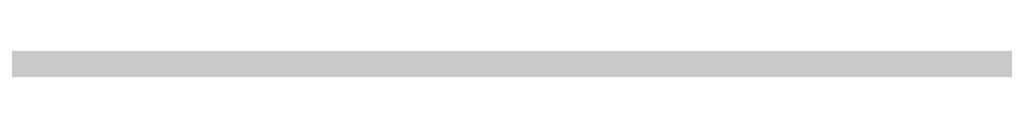
# Model space of a CAD drawing. Units: inches. Extents: x 2091 to 2899, y 967 to 2217.
# Tile 198 of 256: x 2203.18039 to 2203.25707, y 1152.2479 to 1152.24874. Entities that reach past the tile are written whole.
import ezdxf

# ---------------------------------------------------------------- set-up
doc = ezdxf.new("R2010")
doc.units = ezdxf.units.IN
doc.layers.add('A-WALL-PATT', color=141, linetype='Continuous', lineweight=13, true_color=0xadddf7)

msp = doc.modelspace()

# ---------------------------------------------------------------- hatches: boundary and pattern name
at = {"layer": 'A-WALL-PATT'}
h = msp.add_hatch(color=256, dxfattribs=at)
h.dxf.hatch_style = 1
h.paths.add_polyline_path([(2803.143603, 2050.919059), (2203.143603, 2050.919059), (2203.143603, 1090.919059), (2803.143603, 1090.919059)])
h.paths.add_polyline_path([(2635.79885, 1147.540465), (2674.524052, 1147.540465, 0.376086), (2678.529665, 1152.880202), (2678.529665, 1159.556473, 0.333335), (2674.524319, 1163.561846), (2674.524319, 1163.56185), (2674.524319, 1192.93439), (2635.805971, 1192.93439), (2597.087622, 1192.93439), (2597.087622, 1163.561846, 0.333335), (2593.082276, 1159.556473), (2593.082276, 1152.880202, 0.376086), (2597.087889, 1147.540465)], flags=0)
h.paths.add_polyline_path([(2436.010433, 1278.240778, 0.000483), (2435.952643, 1278.215027, -0.001328), (2435.935625, 1278.111693, -0.001711), (2436.11644, 1278.040758, 0.002185)], flags=0)
h.paths.add_polyline_path([(2794.143603, 1143.419059), (2794.143603, 1347.419059), (2543.370171, 1347.419059), (2543.370171, 1351.919059), (2794.143603, 1351.919059), (2794.143603, 1392.713555), (2793.947398, 1392.713555), (2793.947398, 1473.5369), (2794.143603, 1473.5369), (2794.143603, 1531.919059), (2650.143603, 1531.919059), (2650.143603, 1536.419059), (2794.143603, 1536.419059), (2794.143603, 1692.419059), (2609.375609, 1692.419059), (2609.375609, 1644.419059), (2604.875609, 1644.419059), (2604.875609, 1744.919059), (2609.375609, 1744.919059), (2609.375609, 1696.919059), (2794.143603, 1696.919059), (2794.143603, 1780.919059), (2609.643603, 1780.919059), (2493.875609, 1780.919059), (2493.875609, 1785.419059), (2609.643603, 1785.419059), (2794.143603, 1785.419059), (2794.143603, 1847.938821), (2793.951222, 1847.938821), (2793.951222, 1928.762166), (2794.143603, 1928.762166), (2794.143603, 1941.419059), (2614.143603, 1941.419059), (2614.143603, 1821.419059), (2609.643603, 1821.419059), (2609.643603, 1941.419059), (2392.143603, 1941.419059), (2392.143603, 1819.919059), (2387.643603, 1819.919059), (2387.643603, 1941.419059), (2212.143603, 1941.419059), (2212.143603, 1783.919059), (2392.143603, 1783.919059), (2392.143603, 1780.919059), (2212.143603, 1780.919059), (2212.143603, 1629.419059), (2387.643603, 1629.419059), (2387.643603, 1744.919059), (2392.143603, 1744.919059), (2392.143603, 1627.919059), (2317.143603, 1627.919059), (2317.143603, 1551.419059), (2317.143603, 1536.419059), (2459.383591, 1536.419059), (2459.383591, 1602.39648), (2463.883591, 1602.39648), (2463.883591, 1531.919059), (2456.643603, 1531.919059), (2456.643603, 1529.919059), (2452.143603, 1529.919059), (2452.143603, 1531.919059), (2312.643603, 1531.919059), (2312.643603, 1551.419059), (2306.143603, 1551.419059), (2306.143603, 1555.919059), (2308.143603, 1555.919059), (2308.143603, 1551.419059), (2312.643603, 1551.419059), (2312.643603, 1627.919059), (2212.143603, 1627.919059), (2212.143603, 1555.919059), (2270.143603, 1555.919059), (2270.143603, 1551.419059), (2212.143603, 1551.419059), (2212.143603, 1351.919059), (2272.143603, 1351.919059), (2272.143603, 1347.419059), (2212.143603, 1347.419059), (2212.143603, 1275.419059), (2308.143603, 1275.419059), (2308.143603, 1351.919059), (2452.143603, 1351.919059), (2452.143603, 1493.919059), (2456.643603, 1493.919059), (2456.643603, 1347.419059), (2312.643603, 1347.419059), (2312.643603, 1270.919059), (2212.143603, 1270.919059), (2212.143603, 1099.919059), (2281.237523, 1099.919059), (2282.871041, 1110.913803), (2282.008341, 1116.996603), (2278.557741, 1121.420403), (2268.205641, 1128.056203), (2272.087641, 1128.056203), (2273.812941, 1131.927003), (2279.420341, 1134.691903), (2285.027841, 1135.244903), (2287.615841, 1137.456803), (2288.047141, 1138.009803), (2289.341141, 1140.774703), (2291.066541, 1139.668703), (2292.360541, 1135.244903), (2295.379841, 1136.903803), (2296.242541, 1135.797903), (2297.105241, 1133.033003), (2300.124641, 1138.009803), (2303.143941, 1138.009803), (2304.437941, 1135.797903), (2303.143941, 1133.586003), (2306.594641, 1134.691903), (2307.888741, 1133.033003), (2310.908041, 1135.244903), (2313.927441, 1134.138903), (2315.62686, 1132.427102), (2308.320041, 1117.549603), (2290.203841, 1109.807903), (2288.909841, 1103.172103), (2289.272309, 1099.919059), (2434.918227, 1099.919059), (2431.593227, 1124.788059), (2429.930227, 1169.553059), (2430.927185, 1240.519694), (2435.658926, 1238.186126), (2437.135227, 1196.554059), (2438.798227, 1143.973059), (2442.678227, 1111.998059), (2446.558227, 1099.919059), (2794.143603, 1099.919059), (2794.143603, 1138.919059), (2548.032447, 1138.919059), (2548.032447, 1143.419059), (2548.032447, 1148.819059), (2546.668457, 1148.031559), (2528.685692, 1179.178622, 0.256256), (2512.032447, 1148.819059), (2512.032447, 1143.419059), (2512.032447, 1138.919059), (2507.532447, 1138.919059), (2507.532447, 1143.419059), (2507.532447, 1148.819059, 0.256256), (2490.879202, 1179.178622), (2472.896437, 1148.031559), (2471.532447, 1148.819059), (2471.532447, 1143.419059), (2467.032447, 1143.419059), (2467.032447, 1269.945786, 0.039061), (2460.909987, 1273.580059), (2467.032447, 1273.580059), (2467.032447, 1286.325364, 0.014511), (2465.216194, 1286.761905), (2467.032447, 1287.052576), (2467.032447, 1323.419059), (2471.532447, 1323.419059), (2471.532447, 1148.819059), (2489.532447, 1179.995973), (2490.896437, 1179.208473), (2490.879202, 1179.178622, -0.256256), (2507.532447, 1148.819059), (2507.532447, 1143.419059), (2512.032447, 1143.419059), (2512.032447, 1148.819059, -0.256256), (2528.685692, 1179.178622), (2528.668457, 1179.208473), (2530.032447, 1179.995973), (2548.032447, 1148.819059), (2548.032447, 1143.419059)], flags=16)
h.paths.add_polyline_path([(2607.768546, 1200.945083), (2607.768546, 1265.030625), (2597.087622, 1281.052011), (2619.784585, 1281.052011), (2627.795278, 1337.12686), (2635.79885, 1337.12686), (2643.816663, 1337.12686), (2651.827356, 1281.052011), (2674.524319, 1281.052011), (2663.843395, 1265.030625), (2663.843395, 1200.945083), (2635.805971, 1200.945083)], flags=0)
edge = h.paths.add_edge_path(flags=0)
edge.add_ellipse((13303.896215, 1272.998725), major_axis=(-10595.31304, 0.000001), ratio=0.842303870086, start_angle=0.6282372191, end_angle=0.6465540999, ccw=False)
edge.add_ellipse((2711.70045, 1156.852678), major_axis=(2.219769, 0), ratio=0.84230387, start_angle=111.535244, end_angle=180.628237, ccw=False)
edge.add_ellipse((13303.156292, 1272.998725), major_axis=(-10593.026306, 0), ratio=0.842303869544, start_angle=0.5282714718, end_angle=0.6465540971, ccw=False)
edge.add_line((2710.764596, 1175.333295), (2710.129986, 1175.333295))
edge.add_ellipse((2710.129986, 1176.579775), major_axis=(1.479846, 0), ratio=0.84230387, start_angle=180, end_angle=270, ccw=False)
edge.add_line((2708.65014, 1176.579775), (2708.65014, 1200.782914))
edge.add_ellipse((2710.129986, 1200.782914), major_axis=(1.479846, 0), ratio=0.84230387, start_angle=90, end_angle=180, ccw=False)
edge.add_line((2710.129986, 1202.029394), (2710.465075, 1202.029394))
edge.add_ellipse((13303.156292, 1272.998725), major_axis=(-10593.026306, 0), ratio=0.842303869544, start_angle=-0.0902290886, end_angle=0.3838667788, ccw=False)
edge.add_ellipse((2710.129986, 1290.927031), major_axis=(-1.479846, 0), ratio=0.84230387, start_angle=0, end_angle=90, ccw=False)
edge.add_line((2708.65014, 1290.927031), (2708.65014, 1315.13017))
edge.add_ellipse((2710.129986, 1315.13017), major_axis=(-1.479846, 0), ratio=0.84230387, start_angle=-90, end_angle=0, ccw=False)
edge.add_line((2710.129986, 1316.37665), (2710.706314, 1316.37665))
edge.add_ellipse((3238.40172, 1296.289566), major_axis=(528.234, 0), ratio=0.8423038695, start_angle=176.34957241, end_angle=177.82004969, ccw=False)
edge.add_ellipse((2775.063043, 1071.450696), major_axis=(313.307761, 0), ratio=0.8423038695, start_angle=102.12596555, end_angle=103.78052899, ccw=False)
edge.add_ellipse((2775.063043, 1078.305698), major_axis=(-305.302891, 0), ratio=0.8423038695, start_angle=-79.790461, end_angle=-77.55537271, ccw=False)
edge.add_ellipse((2695.141767, 1541.975383), major_axis=(-250.960216, 0), ratio=0.8423038695, start_angle=99.25656601, end_angle=102.55493264)
edge.add_line((2741.410326, 1334.214255), (2747.132545, 1337.378477))
edge.add_ellipse((2747.538616, 1336.857478), major_axis=(-0.739923, 0), ratio=0.8423039, start_angle=270, end_angle=307.93313, ccw=False)
edge.add_ellipse((2747.538616, 1336.857478), major_axis=(-0.739923, 0), ratio=0.8423039, start_angle=232.06687, end_angle=270, ccw=False)
edge.add_line((2747.944687, 1337.378477), (2753.666906, 1334.214255))
edge.add_ellipse((2799.935466, 1541.975383), major_axis=(250.960216, 0), ratio=0.8423038695, start_angle=257.44506736, end_angle=260.74343399)
edge.add_ellipse((2720.014189, 1078.305698), major_axis=(305.302891, 0), ratio=0.8423038695, start_angle=77.55537271, end_angle=79.790461, ccw=False)
edge.add_ellipse((2720.014189, 1071.450696), major_axis=(-313.307761, 0), ratio=0.8423038695, start_angle=256.21947101, end_angle=257.87403445, ccw=False)
edge.add_ellipse((2256.675512, 1296.289566), major_axis=(-528.234, 0), ratio=0.8423038695, start_angle=182.17995031, end_angle=183.65042759, ccw=False)
edge.add_line((2784.370918, 1316.37665), (2784.947247, 1316.37665))
edge.add_ellipse((2784.947247, 1315.13017), major_axis=(1.479846, 0), ratio=0.84230387, start_angle=0, end_angle=90, ccw=False)
edge.add_line((2786.427093, 1315.13017), (2786.427093, 1290.927031))
edge.add_ellipse((2784.947247, 1290.927031), major_axis=(1.479846, 0), ratio=0.84230387, start_angle=270, end_angle=360, ccw=False)
edge.add_ellipse((-7808.07906, 1272.998725), major_axis=(10593.026306, 0), ratio=0.842303869544, start_angle=-0.3838667788, end_angle=0.0902290886, ccw=False)
edge.add_line((2784.612157, 1202.029394), (2784.947247, 1202.029394))
edge.add_ellipse((2784.947247, 1200.782914), major_axis=(1.479846, 0), ratio=0.84230387, start_angle=0, end_angle=90, ccw=False)
edge.add_line((2786.427093, 1200.782914), (2786.427093, 1176.579775))
edge.add_ellipse((2784.947247, 1176.579775), major_axis=(-1.479846, 0), ratio=0.84230387, start_angle=90, end_angle=180, ccw=False)
edge.add_line((2784.947247, 1175.333295), (2784.312636, 1175.333295))
edge.add_ellipse((-7808.07906, 1272.998725), major_axis=(10593.026306, 0), ratio=0.842303869544, start_angle=-0.6186431963, end_angle=-0.5282714718, ccw=False)
edge.add_ellipse((2783.376783, 1156.852678), major_axis=(-2.219769, 0), ratio=0.84230387, start_angle=179.371763, end_angle=248.464757, ccw=False)
edge.add_ellipse((-7808.818983, 1272.998725), major_axis=(-10595.31304, 0.000004), ratio=0.842303865762, start_angle=179.3534459226, end_angle=179.3717628034, ccw=False)
edge.add_ellipse((2780.297303, 1153.500793), major_axis=(-5.246426, 0), ratio=0.84230387, start_angle=90, end_angle=179.353446, ccw=False)
edge.add_line((2780.297303, 1149.081708), (2714.77993, 1149.081708))
edge.add_ellipse((2714.77993, 1153.500793), major_axis=(5.246426, 0), ratio=0.84230387, start_angle=180.646554, end_angle=270, ccw=False)
edge = h.paths.add_edge_path(flags=0)
edge.add_line((2718.187367, 1151.007833), (2718.187367, 1170.472364))
edge.add_ellipse((2721.14706, 1170.472364), major_axis=(-2.959692, 0), ratio=0.84230387, start_angle=-90, end_angle=0, ccw=False)
edge.add_line((2721.14706, 1172.965324), (2773.930173, 1172.965324))
edge.add_ellipse((2773.930173, 1170.472364), major_axis=(-2.959692, 0), ratio=0.84230387, start_angle=180, end_angle=270, ccw=False)
edge.add_line((2776.889865, 1170.472364), (2776.889865, 1151.007833))
edge.add_line((2776.889865, 1151.007833), (2718.187367, 1151.007833))
edge = h.paths.add_edge_path(flags=0)
edge.add_line((2718.187367, 1180.23415), (2718.187367, 1199.057834))
edge.add_ellipse((2747.538616, 1320.39864), major_axis=(147.017924, 0), ratio=0.8423038695, start_angle=256.40186531, end_angle=283.59813469)
edge.add_line((2776.889865, 1199.057834), (2776.889865, 1180.23415))
edge.add_ellipse((2747.538616, 1301.574956), major_axis=(147.017924, 0), ratio=0.8423038695, start_angle=256.40186531, end_angle=283.59813469, ccw=False)
edge = h.paths.add_edge_path(flags=0)
edge.add_ellipse((13303.156292, 1272.998725), major_axis=(-10591.54646, 0), ratio=0.842303869555, start_angle=0.0555943135, end_angle=0.3777641939, ccw=False)
edge.add_line((2711.616859, 1262.72171), (2715.667408, 1249.495396))
edge.add_ellipse((6413.891963, 1241.691919), major_axis=(-3698.236159, 0), ratio=0.84230386955, start_angle=-0.120897369, end_angle=0.364076349)
edge.add_line((2715.761038, 1218.192455), (2711.934307, 1203.167361))
edge = h.paths.add_edge_path(flags=0)
edge.add_line((2718.187367, 1251.074566), (2716.002485, 1267.450435))
edge.add_ellipse((2742.151175, 1202.18954), major_axis=(81.772585, 0), ratio=0.84230387, start_angle=94.27742096, end_angle=111.8349538, ccw=False)
edge.add_line((2737.009748, 1270.930626), (2758.067484, 1270.930626))
edge.add_ellipse((2752.926058, 1202.18954), major_axis=(81.772585, 0), ratio=0.84230387, start_angle=68.1650462, end_angle=85.72257904, ccw=False)
edge.add_line((2779.074747, 1267.450435), (2776.889865, 1251.074566))
edge.add_ellipse((2750.338059, 1187.885356), major_axis=(79.579664, 0), ratio=0.84230387, start_angle=67.20808512, end_angle=85.1299304)
edge.add_line((2756.034656, 1254.743656), (2739.042576, 1254.743656))
edge.add_ellipse((2744.739174, 1187.885356), major_axis=(79.579664, 0), ratio=0.84230387, start_angle=94.8700696, end_angle=112.79191488)
edge = h.paths.add_edge_path(flags=0)
edge.add_line((2783.142926, 1203.167361), (2779.316194, 1218.192455))
edge.add_ellipse((-918.81473, 1241.691919), major_axis=(3698.236159, 0), ratio=0.84230386955, start_angle=-0.364076349, end_angle=0.120897369)
edge.add_line((2779.409825, 1249.495396), (2783.460373, 1262.72171))
edge.add_ellipse((-7808.07906, 1272.998725), major_axis=(-10591.54646, 0), ratio=0.84230386954, start_angle=179.6222358061, end_angle=179.9444056865, ccw=False)
edge = h.paths.add_edge_path(flags=0)
edge.add_ellipse((2734.200892, 1286.69044), major_axis=(-0.356609, 6.340078), ratio=0.60383358, start_angle=89.0020143, end_angle=253.657408, ccw=False)
edge.add_line((2730.369001, 1286.541806), (2730.369001, 1301.35198))
edge.add_line((2730.369001, 1301.35198), (2735.913311, 1305.214803))
edge.add_ellipse((2736.384917, 1304.734561), major_axis=(0.739923, 0), ratio=0.8423039, start_angle=90, end_angle=134.480211, ccw=False)
edge.add_line((2736.384917, 1305.357801), (2738.032783, 1305.357801))
edge.add_line((2738.032783, 1305.357801), (2738.032783, 1307.707927))
edge.add_ellipse((2794.201642, 1307.707927), major_axis=(56.168859, 0), ratio=0.84230387, start_angle=150.5614304, end_angle=180, ccw=False)
edge.add_ellipse((2700.875591, 1307.707927), major_axis=(-56.168859, 0), ratio=0.84230387, start_angle=180, end_angle=209.4385696, ccw=False)
edge.add_line((2757.04445, 1307.707927), (2757.04445, 1305.357801))
edge.add_line((2757.04445, 1305.357801), (2758.692316, 1305.357801))
edge.add_ellipse((2758.692316, 1304.734561), major_axis=(-0.739923, 0), ratio=0.8423039, start_angle=225.519789, end_angle=270, ccw=False)
edge.add_line((2759.163922, 1305.214803), (2764.708231, 1301.35198))
edge.add_line((2764.708231, 1301.35198), (2764.708231, 1286.541806))
edge.add_ellipse((2760.87634, 1286.69044), major_axis=(0.356609, 6.340078), ratio=0.60383358, start_angle=106.342592, end_angle=270.9979857, ccw=False)
edge.add_line((2757.04445, 1285.79709), (2757.04445, 1307.707927))
edge.add_ellipse((2700.875591, 1307.707927), major_axis=(-56.168859, 0), ratio=0.84230387, start_angle=180, end_angle=209.4385696)
edge.add_ellipse((2794.201642, 1307.707927), major_axis=(56.168859, 0), ratio=0.84230387, start_angle=150.5614304, end_angle=180)
edge.add_line((2738.032783, 1307.707927), (2738.032783, 1285.79709))
h.paths.add_polyline_path([(2417.812273, 1104.449704), (2413.492273, 1102.529704), (2410.612273, 1103.969704), (2409.172273, 1106.369704), (2407.252273, 1107.329704), (2406.292273, 1109.729704), (2405.332273, 1114.049704), (2405.332273, 1117.889704), (2406.292273, 1120.129704), (2407.252273, 1119.809704), (2408.848322, 1118.327658), (2410.173945, 1119.42417), (2410.211273, 1120.405704), (2411.040731, 1121.419054), (2410.699273, 1119.858704), (2410.173945, 1119.42417), (2410.088452, 1117.176109), (2411.132836, 1116.206324), (2413.972273, 1119.329704), (2416.852273, 1120.769704), (2416.869721, 1120.798784), (2417.035071, 1119.405116), (2417.896213, 1118.143384), (2418.292273, 1118.369704), (2419.544447, 1120.039269), (2419.360915, 1118.387487), (2419.032108, 1119.356151), (2418.398939, 1118.511926), (2419.252273, 1114.529704), (2418.794091, 1107.198795)], flags=0)
h.paths.add_polyline_path([(2508.870171, 1347.419059), (2508.370171, 1347.419059), (2508.370171, 1351.919059), (2508.870171, 1351.919059)], flags=0)
h.paths.add_polyline_path([(2473.370171, 1347.419059), (2472.370171, 1347.419059), (2467.870171, 1347.419059), (2467.870171, 1455.419059), (2472.370171, 1455.419059), (2472.370171, 1352.419059), (2473.370171, 1352.419059)], flags=0)
h.paths.add_polyline_path([(2352.106244, 1217.446197), (2349.226244, 1218.886197), (2347.786244, 1221.286197), (2345.866244, 1222.246197), (2344.906244, 1224.646197), (2343.946244, 1228.966197), (2343.946244, 1232.806197), (2344.906244, 1235.046197), (2345.866244, 1234.726197), (2347.462293, 1233.244152), (2348.787916, 1234.340663), (2348.825244, 1235.322197), (2349.654702, 1236.335547), (2349.313244, 1234.775197), (2348.787916, 1234.340663), (2348.702423, 1232.092603), (2349.746807, 1231.122817), (2352.586244, 1234.246197), (2355.466244, 1235.686197), (2355.483692, 1235.715277), (2355.649043, 1234.321609), (2356.510185, 1233.059877), (2356.906244, 1233.286197), (2358.158418, 1234.955762), (2357.974887, 1233.30398), (2357.646079, 1234.272644), (2357.012911, 1233.428419), (2357.866244, 1229.446197), (2357.408062, 1222.115288), (2356.426244, 1219.366197)], flags=0)
h.paths.add_polyline_path([(2348.2968, 1112.22442), (2347.0138, 1112.31042), (2345.5298, 1114.12742), (2345.7318, 1115.85842), (2346.8118, 1116.98242), (2346.8118, 1114.64642), (2345.8668, 1114.21442), (2346.8798, 1114.30042)], flags=0)
h.paths.add_polyline_path([(2347.0138, 1110.92642), (2346.2718, 1110.49342), (2346.6098, 1111.18642)], flags=0)
h.paths.add_polyline_path([(2345.8668, 1118.19442), (2345.5298, 1117.32942), (2343.7078, 1118.02142), (2344.3828, 1118.62642)], flags=0)
h.paths.add_polyline_path([(2346.6768, 1109.28242), (2346.0698, 1108.07142), (2345.8668, 1110.06142)], flags=0)
h.paths.add_polyline_path([(2345.0568, 1119.75142), (2343.6398, 1119.75142), (2343.9778, 1121.13542)], flags=0)
h.paths.add_polyline_path([(2345.2598, 1116.55042), (2345.1248, 1115.85842), (2344.9218, 1115.68542), (2344.7198, 1116.37742)], flags=0)
h.paths.add_polyline_path([(2345.6648, 1112.31042), (2345.4618, 1111.53242), (2344.0448, 1111.96442), (2344.6518, 1112.57042)], flags=0)
h.paths.add_polyline_path([(2345.1918, 1113.34942), (2344.4498, 1113.86842), (2344.7198, 1114.38742)], flags=0)
h.paths.add_polyline_path([(2344.6518, 1116.80942), (2344.1798, 1115.68542), (2344.6518, 1115.33942), (2343.9098, 1114.90642), (2343.0328, 1115.94442), (2343.6398, 1116.46342)], flags=0)
h.paths.add_polyline_path([(2345.8668, 1106.68642), (2344.9898, 1105.56242), (2344.5168, 1106.60042)], flags=0)
h.paths.add_polyline_path([(2344.8548, 1110.06142), (2344.5168, 1109.28242), (2344.1128, 1109.71542)], flags=0)
h.paths.add_polyline_path([(2344.0448, 1113.52242), (2343.4378, 1113.08942), (2342.7628, 1113.95442)], flags=0)
h.paths.add_polyline_path([(2344.3148, 1111.01242), (2342.9648, 1110.32042), (2342.9648, 1111.09942)], flags=0)
h.paths.add_polyline_path([(2345.1248, 1104.69742), (2344.5848, 1103.74542), (2344.4498, 1104.26442)], flags=0)
h.paths.add_polyline_path([(2342.8298, 1121.22242), (2341.7498, 1120.53042), (2340.5358, 1121.04942), (2340.1308, 1121.82842), (2340.6708, 1122.95242), (2341.1428, 1121.82842), (2341.6148, 1122.00142)], flags=0)
h.paths.add_polyline_path([(2342.9648, 1119.75142), (2343.0328, 1118.45342), (2342.0878, 1118.02142), (2342.0198, 1119.49142)], flags=0)
h.paths.add_polyline_path([(2342.6948, 1116.89642), (2341.9528, 1116.63642), (2342.0198, 1117.32942)], flags=0)
h.paths.add_polyline_path([(2343.0328, 1112.22442), (2342.0198, 1111.79142), (2341.5478, 1112.22442), (2342.3578, 1113.34942)], flags=0)
h.paths.add_polyline_path([(2343.7748, 1104.43742), (2342.6278, 1102.88042), (2342.6948, 1104.61042), (2343.4378, 1105.12942)], flags=0)
h.paths.add_polyline_path([(2342.0198, 1115.07942), (2340.8058, 1115.51242), (2340.9408, 1116.37742)], flags=0)
h.paths.add_polyline_path([(2341.4808, 1120.09742), (2341.4808, 1119.40542), (2341.0758, 1119.57842), (2341.1428, 1120.09742)], flags=0)
h.paths.add_polyline_path([(2341.8178, 1114.47342), (2340.9408, 1113.08942), (2340.8058, 1114.56042)], flags=0)
h.paths.add_polyline_path([(2341.1428, 1118.54042), (2340.9408, 1116.98242), (2339.0508, 1117.67542), (2339.0508, 1118.62642)], flags=0)
h.paths.add_polyline_path([(2342.6948, 1101.66842), (2341.9528, 1101.84142), (2342.5598, 1102.36142)], flags=0)
h.paths.add_polyline_path([(2340.3328, 1119.66542), (2338.4438, 1119.57842), (2337.9038, 1120.35742), (2339.6578, 1120.61642)], flags=0)
h.paths.add_polyline_path([(2340.3328, 1115.33942), (2340.0628, 1113.69542), (2339.3878, 1115.33942)], flags=0)
h.paths.add_polyline_path([(2341.8178, 1103.83142), (2341.5478, 1102.88042), (2341.1428, 1103.65842)], flags=0)
h.paths.add_polyline_path([(2339.0508, 1122.86642), (2337.2958, 1121.82842), (2337.0938, 1123.12542), (2337.7688, 1123.81842)], flags=0)
h.paths.add_polyline_path([(2339.1178, 1121.74142), (2338.8478, 1121.22242), (2338.1738, 1121.04942), (2338.3758, 1121.56842)], flags=0)
h.paths.add_polyline_path([(2339.1858, 1119.31942), (2338.6458, 1118.71342), (2338.2408, 1118.10742), (2338.2408, 1118.88642)], flags=0)
h.paths.add_polyline_path([(2341.1428, 1101.92842), (2340.6028, 1101.23642), (2340.0628, 1101.84142), (2340.6028, 1102.36142)], flags=0)
h.paths.add_polyline_path([(2337.6338, 1117.76142), (2336.6208, 1118.28042), (2337.2958, 1118.97242)], flags=0)
h.paths.add_polyline_path([(2336.8238, 1119.57842), (2334.7988, 1118.97242), (2335.2038, 1120.35742), (2336.5538, 1120.87642)], flags=0)
h.paths.add_polyline_path([(2339.1178, 1100.45742), (2337.3638, 1100.54342), (2336.7558, 1101.23642)], flags=0)
h.paths.add_polyline_path([(2336.3508, 1122.43342), (2336.0138, 1121.91442), (2334.9338, 1122.43342), (2334.5288, 1123.47142), (2335.7438, 1122.77942)], flags=0)
h.paths.add_polyline_path([(2334.7318, 1120.87642), (2334.2588, 1120.35742), (2334.0568, 1120.78942), (2334.5968, 1121.30842)], flags=0)
h.paths.add_polyline_path([(2334.4618, 1122.17442), (2332.5718, 1121.30842), (2331.3568, 1122.17442), (2332.0998, 1122.86642)], flags=0)
h.paths.add_polyline_path([(2334.2588, 1118.54042), (2333.3818, 1118.45342), (2333.6518, 1119.31942)], flags=0)
h.paths.add_polyline_path([(2335.5418, 1102.27442), (2334.1918, 1102.62042), (2335.2718, 1103.31242)], flags=0)
h.paths.add_polyline_path([(2332.7068, 1119.66542), (2331.6948, 1120.44342), (2332.5048, 1120.78942)], flags=0)
h.paths.add_polyline_path([(2334.7318, 1101.14942), (2333.5168, 1101.58242), (2333.9888, 1101.75542)], flags=0)
h.paths.add_polyline_path([(2332.6398, 1116.63642), (2331.0868, 1116.29042), (2331.9648, 1118.19442)], flags=0)
h.paths.add_polyline_path([(2330.7498, 1121.56842), (2330.2768, 1120.27042), (2328.5228, 1119.31942), (2328.9948, 1121.04942)], flags=0)
h.paths.add_polyline_path([(2330.7498, 1118.62642), (2330.0078, 1117.50242), (2329.8728, 1118.02142)], flags=0)
h.paths.add_polyline_path([(2332.0998, 1102.36142), (2330.5468, 1102.01442), (2331.6948, 1102.96642)], flags=0)
h.paths.add_polyline_path([(2329.5348, 1113.60842), (2329.0628, 1112.31042), (2328.5898, 1113.34942)], flags=0)
h.paths.add_polyline_path([(2328.3878, 1117.84842), (2327.5098, 1116.55042), (2327.1728, 1117.76142)], flags=0)
h.paths.add_polyline_path([(2329.7378, 1106.51342), (2329.5348, 1105.30242), (2328.2528, 1106.08142)], flags=0)
h.paths.add_polyline_path([(2328.6578, 1114.38742), (2328.0498, 1114.12742), (2328.3198, 1114.90642)], flags=0)
h.paths.add_polyline_path([(2328.3198, 1112.22442), (2327.1058, 1112.13742), (2326.7008, 1112.65642)], flags=0)
h.paths.add_polyline_path([(2326.9028, 1115.25242), (2326.7008, 1114.12742), (2325.2158, 1113.60842), (2326.0928, 1115.33942)], flags=0)
h.paths.add_polyline_path([(2326.6328, 1108.33042), (2326.0928, 1107.37942), (2325.8908, 1108.50342), (2326.4978, 1109.10942)], flags=0)
h.paths.add_polyline_path([(2615.143603, 1531.919059), (2609.643603, 1531.919059), (2609.643603, 1620.419059), (2614.143603, 1620.419059), (2614.143603, 1536.419059), (2615.143603, 1536.419059)], flags=0)
h.paths.add_polyline_path([(2545.143603, 1563.419059), (2464.143603, 1563.419059), (2464.143603, 1632.419059), (2509.143603, 1632.419059), (2509.143603, 1627.919059), (2509.143603, 1603.919059), (2468.643603, 1603.919059), (2468.643603, 1567.919059), (2540.643603, 1567.919059), (2540.643603, 1591.919059), (2545.143603, 1591.919059)], flags=0)
h.paths.add_polyline_path([(2388.969048, 1549.985735), (2357.434181, 1549.985735), (2357.434181, 1623.360778), (2399.362777, 1623.360778), (2435.689465, 1623.360778), (2435.592547, 1602.559273), (2435.592547, 1602.39648), (2388.969048, 1602.39648)], flags=0)
h.paths.add_polyline_path([(2388.880628, 1555.809151), (2374.904429, 1555.809151), (2374.904429, 1600.571564), (2374.904429, 1615.457645), (2406.350877, 1615.457645), (2406.350877, 1618.939431), (2412.174293, 1615.457645), (2406.350877, 1611.97586), (2406.350877, 1615.457645), (2388.880628, 1615.457645)], flags=0)
h.paths.add_polyline_path([(2568.875609, 1644.419059), (2453.375609, 1644.419059), (2453.375609, 1785.419059), (2457.875609, 1785.419059), (2457.875609, 1648.919059), (2568.875609, 1648.919059)], flags=0)
h.paths.add_polyline_path([(2212.143603, 1945.919059), (2212.143603, 2041.919059), (2794.143603, 2041.919059), (2794.143603, 1945.919059)], flags=16)
h.paths.add_polyline_path([(2271.082728, 1964.317238), (2776.852968, 1964.317238), (2776.852968, 2037.169623), (2271.082728, 2037.169623)], flags=8)
h.paths.add_polyline_path([(2380.649285, 1536.824144), (2461.040809, 1536.824144), (2461.040809, 1554.652587), (2380.649285, 1554.652587)], flags=8)
h.paths.add_polyline_path([(2240.755709, 1609.725451), (2309.185829, 1609.725451), (2309.185829, 1617.698204), (2240.755709, 1617.698204)], flags=8)
h.paths.add_polyline_path([(2212.677255, 1313.504102), (2282.59152, 1313.504102), (2282.59152, 1322.745239), (2212.677255, 1322.745239)], flags=8)
h.paths.add_polyline_path([(2457.111976, 1114.778574), (2558.481581, 1114.778574), (2558.481581, 1142.219682), (2457.111976, 1142.219682)], flags=8)
h.paths.add_polyline_path([(2473.442337, 1273.010067), (2604.641226, 1273.010067), (2604.641226, 1318.346935), (2473.442337, 1318.346935)], flags=8)
h.paths.add_polyline_path([(2638.876302, 1626.977432), (2684.250367, 1627.976738), (2684.038483, 1637.597494), (2638.664417, 1636.598188)], flags=8)
h.paths.add_polyline_path([(2537.590554, 1453.793447), (2628.389547, 1453.793447), (2628.389547, 1475.344811), (2537.590554, 1475.344811)], flags=8)
h.paths.add_polyline_path([(2504.137638, 1714.632397), (2554.647187, 1714.632397), (2554.647187, 1730.237712), (2504.137638, 1730.237712)], flags=8)
h.paths.add_polyline_path([(2487.501181, 1575.651872), (2535.097121, 1575.651872), (2535.097121, 1598.377646), (2487.501181, 1598.377646)], flags=8)
h.paths.add_polyline_path([(2709.0994, 1735.710278), (2740.016601, 1735.710278), (2740.016601, 1749.937641), (2709.0994, 1749.937641)], flags=8)
h.paths.add_polyline_path([(2442.438424, 1792.171657), (2564.728835, 1792.171657), (2564.728835, 1842.000163), (2442.438424, 1842.000163)], flags=8)
h.paths.add_polyline_path([(2655.815801, 1809.644076), (2789.520142, 1806.693796), (2790.084977, 1832.291638), (2656.380635, 1835.241918)], flags=8)
h.paths.add_polyline_path([(2234.842697, 1797.720143), (2368.592851, 1794.768852), (2369.160718, 1820.504132), (2235.410564, 1823.455423)], flags=8)
h.paths.add_polyline_path([(2245.138466, 1644.006335), (2398.427733, 1640.6239), (2398.994842, 1666.32482), (2245.705575, 1669.707255)], flags=8)
h.paths.add_polyline_path([(2306.142847, 1431.168519), (2413.768314, 1428.793687), (2414.333148, 1454.391529), (2306.707682, 1456.76636)], flags=8)
h.paths.add_polyline_path([(2306.834582, 1458.233145), (2393.380484, 1456.323449), (2393.932808, 1481.354358), (2307.386907, 1483.264054)], flags=8)

doc.saveas('drawing.dxf')
